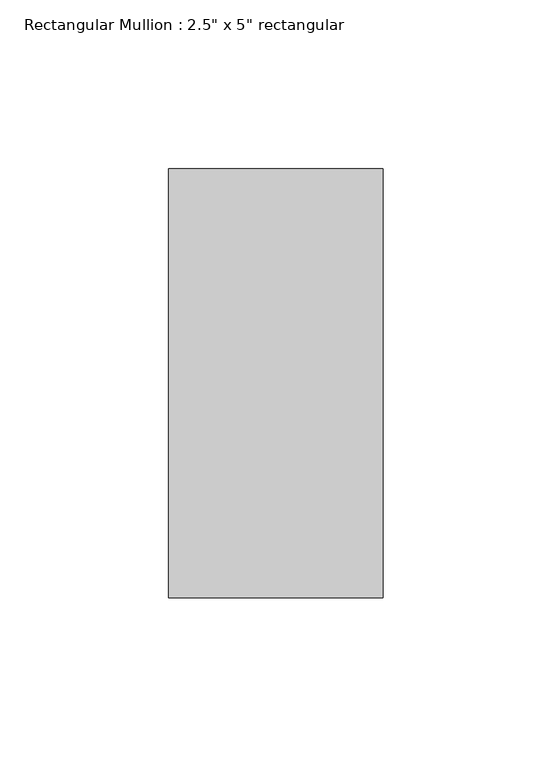
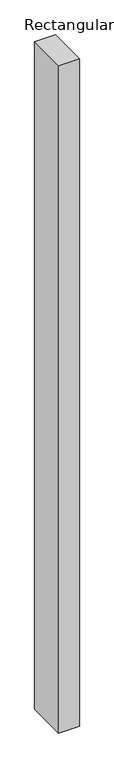
"""IFC4 building model written with IfcOpenShell, lengths in millimetres: member geometry."""

from ifc_helpers import new_model, si_unit, frame, origin, place, context, project, spatial, polyline, outline, extrude, source, transform, mapped, element, save


def member_e9262278(model_context):
    return source(origin(), model_context, "Body", "SweptSolid", [
        extrude(outline(polyline([(0.0, 63.5), (0.0, -63.5), (-63.5, -63.5), (-63.5, 63.5), (0.0, 63.5)])), frame((0.0, 0.0, -2161.4673659), z_axis=(0.0, 0.0, 1.0), x_axis=(1.0, 0.0, 0.0)), (0.0, 0.0, 1.0), 2161.4673659),
    ])


if __name__ == "__main__":
    model = new_model("IFC4")
    model_context = context("Model", 3, world=origin())
    ifc_project = project(units=[si_unit("LENGTHUNIT", "METRE", prefix="MILLI")], contexts=[model_context])
    site = spatial("IfcSite", under=ifc_project)
    building = spatial("IfcBuilding", under=site)
    placement = place(None, origin())
    member_shape = member_e9262278(model_context)
    element("IfcMember", 1, ObjectType="Rectangular Mullion : 2.5\" x 5\" rectangular", at=placement, inside=building, context=model_context, shape_type="MappedRepresentation", body=[
        mapped(member_shape, transform((0.0, 0.0, 0.0), x_axis=(1.0, 0.0, 0.0), y_axis=(0.0, 1.0, 0.0), z_axis=(0.0, 0.0, 1.0))),
    ])
    save(model, "model.ifc")

# Revit data of these elements
# Type "Rectangular Mullion : 2.5\" x 5\" rectangular"
#   built-in parameter 1007304 = 0.416667 (stored number, unit not read)
#   built-in parameter 1007301 = 0.104167 (stored number, unit not read)
#   built-in parameter 1007300 = 0.104167 (stored number, unit not read)
# Element 1 (IfcMember, "Rectangular Mullion : 2.5\" x 5\" rectangular")
#   Materials on its faces: "Aluminum"
# Materials
#   "Aluminum": class "Metal", colour RGB 247 247 247, transparency 0, Description = "Aluminum 6061", Cost = 0
